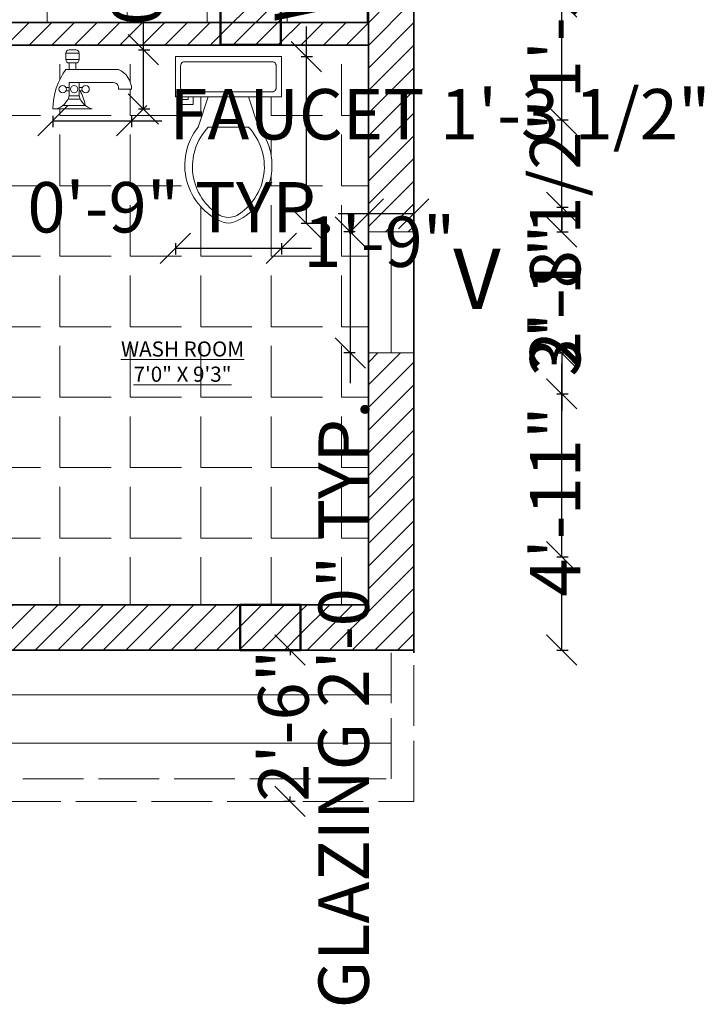
# Model space of a CAD drawing. Units: inches. Extents: x 2036 to 2670, y 319 to 920.
# Tile 13 of 15: x 2535 to 2670, y 424 to 620. Entities that reach past the tile are written whole.
import ezdxf

# ---------------------------------------------------------------- set-up
doc = ezdxf.new("R2010")
doc.units = ezdxf.units.IN
doc.linetypes.add('ACAD_ISO02W100', pattern=[15, 12, -3])
for name, color, linetype, lineweight in [('A-ANNO-DIMS', 2, 'Continuous', 18), ('A-ANNO-TEXT', 7, 'Continuous', 18), ('A-AREA-IDEN', 7, 'Continuous', 18), ('A-COLS', 7, 'Continuous', 50), ('A-FLOR-FIXT', 8, 'Continuous', 18), ('A-FLOR-OVHD', 1, 'ACAD_ISO02W100', 13), ('A-FLOR-PATT', 8, 'Continuous', 9), ('A-GLAZ', 4, 'Continuous', 18), ('A-WALL', 7, 'Continuous', 35)]:
    doc.layers.add(name, color=color, linetype=linetype, lineweight=lineweight)
doc.layers.add('A-COLS-PATT', color=240, linetype='Continuous', lineweight=13, true_color=0xed1f24)
doc.layers.add('A-WALL-PATT', color=52, linetype='Continuous', lineweight=13, true_color=0xc8c92d)
doc.styles.get("Standard").update_dxf_attribs({"font": 'arial.ttf'})
doc.dimstyles.new('ISO-25', dxfattribs={"dimtxt": 10, "dimasz": 6, "dimexe": 1.25, "dimexo": 0.625, "dimtad": 0, "dimdec": 1, "dimlunit": 3, "dimtxsty": 'Standard', "dimblk": 'OBLIQUE', "dimcen": 2.5, "dimclrd": 94, "dimclre": 94, "dimclrt": 1, "dimadec": 0, "dimazin": 0, "dimtfac": 1, "dimtdec": 1, "dimtmove": 0, "dimatfit": 3, "dimfxl": 1, "dimfxlon": 1, "dimarcsym": 0})

# ---------------------------------------------------------------- blocks, each defined once
blk = doc.blocks.new('Toilet - top')
for p, q in [((9.5, -6), (9.5, -2)), ((-10, -8.5), (-8, -8.5)), ((-10, -9.5), (-10, -8.5)), ((-7, -9.5), (-10, -9.5)), ((-8, -8.5), (-8, -8)), ((-7, -8), (-7, -9.5)), ((-4, -8), (-6, -14)), ((4, -8), (6, -14)), ((4, -14), (-4, -14))]:
    blk.add_line(p, q)
blk.add_lwpolyline([(10.5, -8), (10.5, 0), (-10.5, 0), (-10.5, -8)], close=True)
for points in [[(8.5, -1), (-8.5, -1)], [(-9.5, -2), (-9.5, -6)], [(-8.5, -7), (8.5, -7)]]:
    blk.add_lwpolyline(points)
for centre, radius, start, end in [((-8.62, -1.88), 0.884, 81.8699, 188.1301), ((8.62, -1.88), 0.884, 351.8699, 98.1301), ((-8.62, -6.12), 0.884, 171.8699, 278.1301), ((8.62, -6.12), 0.884, 261.8699, 8.1301), ((3.52, -21.58), 12.17, 141.4691, 247.9714), ((4.2, -21.82), 11.33, 136.3677, 238.9468), ((-3.52, -21.58), 12.17, 292.0284, 38.5307), ((-4.2, -21.82), 11.33, 301.053, 43.6321), ((0, -27.88), 4, 245.7318, 294.2682), ((0, -29), 4, 254.8605, 285.1395)]:
    blk.add_arc(centre, radius, start, end)
blk = doc.blocks.new('Faucet - Bathroom side')
for p, q in [((-0.625, 4.25), (0.375, 4.25)), ((0.375, 3.75), (-0.625, 3.75)), ((-0.625, 3), (3.375, 3)), ((-0.375, 3), (-0.375, 3.5)), ((0.125, 3.5), (0.125, 3)), ((-0.375, 1.625), (-0.625, 1.625)), ((2.875, 2), (0.375, 2)), ((0.375, 1.625), (0.625, 1.625)), ((4.375, 1.5), (3.375, 1.5)), ((-0.375, 1.375), (-0.625, 1.375)), ((0.48078, 0.75), (-0.47286, 0.75)), ((0.375, 1.375), (0.625, 1.375)), ((-1.625, 0), (-1.375, 0)), ((-1.375, 0), (1.375, 0)), ((-0.88366, 0.25), (0.88424, 0.25))]:
    blk.add_line(p, q)
for points in [[(-0.375, 4.5), (0.125, 4.5)], [(-0.625, 3.75), (-0.625, 4.25)], [(0.375, 4.25), (0.375, 3.75)], [(0.125, 3.5), (-0.375, 3.5)]]:
    blk.add_lwpolyline(points)
blk.add_lwpolyline([(-0.375, 1), (-0.375, 2), (0.375, 2), (0.375, 1)], close=True)
for centre in [(-0.875, 1.5), (0, 1.5), (0.875, 1.5)]:
    blk.add_circle(centre, 0.27951)
for centre, radius, start, end in [((-0.38253, 4.2575), 0.24259, 88.22243, 181.7776), ((0.13252, 4.2575), 0.24259, 358.2224, 91.77757), ((-0.38253, 3.7424), 0.24259, 178.2224, 271.7776), ((0.13252, 3.7424), 0.24259, 268.2224, 1.777565), ((3.45929, -0.0281), 5.08436, 143.4467, 179.6834), ((2.70708, 1.4714), 1.66816, 0.9827695, 66.39737), ((2.96867, 1.5936), 0.41699, 347.0192, 102.9808), ((-1.75, 1.375), 1.42522, 285.2551, 344.7449), ((1.75, 1.375), 1.42522, 195.2551, 254.7449), ((-2.49562, -0.286), 3.38273, 9.709485, 29.48735)]:
    blk.add_arc(centre, radius, start, end)
blk = doc.blocks.new('_Oblique')
at = {"color": 0, "linetype": 'ByBlock', "lineweight": -2}
blk.add_line((-0.5, -0.5), (0.5, 0.5), dxfattribs=at)
blk = doc.blocks.new('*D12')
at = {"layer": 'A-ANNO-DIMS', "color": 0, "lineweight": -2, "transparency": 16777216}
for p, q in [((2589.2, 494.68), (2586.95, 494.68)), ((2588.2, 494.68), (2588.2, 493.69)), ((2588.2, 464.68), (2588.2, 465.68)), ((2589.2, 464.68), (2586.95, 464.68))]:
    blk.add_line(p, q, dxfattribs=at)
at = {"layer": 'Defpoints', "color": 0, "transparency": 16777216}
for p in [(2588.2, 494.68), (2612.74, 494.68), (2612.74, 464.68)]:
    blk.add_point(p, dxfattribs=at)
at = {"layer": 'A-ANNO-DIMS', "color": 0, "lineweight": -2, "transparency": 16777216, "xscale": 6, "yscale": 6, "zscale": 6}
for p, rotation in [((2588.2, 494.68), 90), ((2588.2, 464.68), 270)]:
    blk.add_blockref('_Oblique', p, dxfattribs=dict(at, rotation=rotation))
at = {"layer": 'A-ANNO-DIMS', "color": 0, "transparency": 16777216, "insert": (2588.2, 479.68), "char_height": 10, "attachment_point": 5, "rotation": 90}
blk.add_mtext('2\'-6"', dxfattribs=at)
blk = doc.blocks.new('COL-9x12')
blk.add_lwpolyline([(9, 0), (0, 0), (0, 12), (9, 12)], close=True)
blk = doc.blocks.new('GLAZ-24x9-PLAN')
for p, q in [((9, 24), (0, 24)), ((4.5, 24), (4.5, 0)), ((9, 0), (0, 0))]:
    blk.add_line(p, q)
blk = doc.blocks.new('*D29')
at = {"layer": 'A-ANNO-DIMS', "color": 94, "lineweight": -2, "transparency": 16777216}
for p, q in [((2601.14, 577.61), (2598.89, 577.61)), ((2600.14, 577.61), (2600.14, 553.61)), ((2601.14, 553.61), (2598.89, 553.61)), ((2600.14, 553.61), (2600.14, 547.61))]:
    blk.add_line(p, q, dxfattribs=at)
at = {"layer": 'Defpoints', "color": 0, "transparency": 16777216}
for p in [(2603.74, 577.61), (2600.14, 553.61), (2603.74, 553.61)]:
    blk.add_point(p, dxfattribs=at)
at = {"layer": 'A-ANNO-DIMS', "color": 94, "lineweight": -2, "transparency": 16777216, "xscale": 6, "yscale": 6, "zscale": 6}
for p, rotation in [((2600.14, 577.61), 90), ((2600.14, 553.61), 270)]:
    blk.add_blockref('_Oblique', p, dxfattribs=dict(at, rotation=rotation))
at = {"layer": 'A-ANNO-DIMS', "color": 1, "transparency": 16777216, "insert": (2600.14, 483.98), "char_height": 10, "attachment_point": 5, "rotation": 90}
blk.add_mtext('GLAZING 2\'-0" TYP.', dxfattribs=at)
blk = doc.blocks.new('*D30')
at = {"layer": 'A-ANNO-DIMS', "color": 94, "lineweight": -2, "transparency": 16777216}
for p, q in [((2603.74, 580.21), (2603.74, 582.46)), ((2612.74, 580.21), (2612.74, 582.46)), ((2603.74, 581.21), (2597.74, 581.21)), ((2612.74, 581.21), (2603.74, 581.21))]:
    blk.add_line(p, q, dxfattribs=at)
at = {"layer": 'Defpoints', "color": 0, "transparency": 16777216}
for p in [(2603.74, 581.21), (2603.74, 577.61), (2612.74, 577.61)]:
    blk.add_point(p, dxfattribs=at)
at = {"layer": 'A-ANNO-DIMS', "color": 94, "lineweight": -2, "transparency": 16777216, "xscale": 6, "yscale": 6, "zscale": 6, "rotation": 180}
blk.add_blockref('_Oblique', (2603.74, 581.21), dxfattribs=at)
at = {"layer": 'A-ANNO-DIMS', "color": 94, "lineweight": -2, "transparency": 16777216, "xscale": 6, "yscale": 6, "zscale": 6}
blk.add_blockref('_Oblique', (2612.74, 581.21), dxfattribs=at)
at = {"layer": 'A-ANNO-DIMS', "color": 1, "transparency": 16777216, "insert": (2566.63, 581.21), "char_height": 10, "attachment_point": 5}
blk.add_mtext('0\'-9" TYP.', dxfattribs=at)
blk = doc.blocks.new('*D35')
at = {"layer": 'A-ANNO-DIMS', "color": 94, "lineweight": -2, "transparency": 16777216}
for p, q in [((2591.44, 612.38), (2591.44, 618.38)), ((2590.44, 612.38), (2592.69, 612.38)), ((2591.44, 579.34), (2591.44, 612.38)), ((2590.44, 579.34), (2592.69, 579.34))]:
    blk.add_line(p, q, dxfattribs=at)
at = {"layer": 'Defpoints', "color": 0, "transparency": 16777216}
for p in [(2586.48, 612.38), (2591.44, 612.38), (2586.48, 579.34)]:
    blk.add_point(p, dxfattribs=at)
at = {"layer": 'A-ANNO-DIMS', "color": 94, "lineweight": -2, "transparency": 16777216, "xscale": 6, "yscale": 6, "zscale": 6}
for p, rotation in [((2591.44, 612.38), 90), ((2591.44, 579.34), 270)]:
    blk.add_blockref('_Oblique', p, dxfattribs=dict(at, rotation=rotation))
at = {"layer": 'A-ANNO-DIMS', "color": 1, "transparency": 16777216, "insert": (2591.44, 646.08), "char_height": 10, "attachment_point": 5, "rotation": 90}
blk.add_mtext('WC 2\'-9"', dxfattribs=at)
blk = doc.blocks.new('*D36')
at = {"layer": 'A-ANNO-DIMS', "color": 94, "lineweight": -2, "transparency": 16777216}
for p, q in [((2565.48, 575.38), (2565.48, 573.13)), ((2565.48, 574.38), (2586.48, 574.38)), ((2586.48, 575.38), (2586.48, 573.13)), ((2586.48, 574.38), (2592.48, 574.38))]:
    blk.add_line(p, q, dxfattribs=at)
at = {"layer": 'Defpoints', "color": 0, "transparency": 16777216}
for p in [(2565.48, 579.34), (2586.48, 579.34), (2586.48, 574.38)]:
    blk.add_point(p, dxfattribs=at)
at = {"layer": 'A-ANNO-DIMS', "color": 94, "lineweight": -2, "transparency": 16777216, "xscale": 6, "yscale": 6, "zscale": 6, "rotation": 180}
blk.add_blockref('_Oblique', (2565.48, 574.38), dxfattribs=at)
at = {"layer": 'A-ANNO-DIMS', "color": 94, "lineweight": -2, "transparency": 16777216, "xscale": 6, "yscale": 6, "zscale": 6}
blk.add_blockref('_Oblique', (2586.48, 574.38), dxfattribs=at)
at = {"layer": 'A-ANNO-DIMS', "color": 1, "transparency": 16777216, "insert": (2605.93, 574.38), "char_height": 10, "attachment_point": 5}
blk.add_mtext('1\'-9"', dxfattribs=at)
blk = doc.blocks.new('*D37')
at = {"layer": 'A-ANNO-DIMS', "color": 94, "lineweight": -2, "transparency": 16777216}
for p, q in [((2541.16, 600.66), (2541.16, 598.41)), ((2541.16, 599.66), (2556.79, 599.66)), ((2556.79, 600.66), (2556.79, 598.41)), ((2556.79, 599.66), (2562.79, 599.66))]:
    blk.add_line(p, q, dxfattribs=at)
at = {"layer": 'Defpoints', "color": 0, "transparency": 16777216}
for p in [(2541.16, 602.01), (2556.79, 602.01), (2556.79, 599.66)]:
    blk.add_point(p, dxfattribs=at)
at = {"layer": 'A-ANNO-DIMS', "color": 94, "lineweight": -2, "transparency": 16777216, "xscale": 6, "yscale": 6, "zscale": 6, "rotation": 180}
blk.add_blockref('_Oblique', (2541.16, 599.66), dxfattribs=at)
at = {"layer": 'A-ANNO-DIMS', "color": 94, "lineweight": -2, "transparency": 16777216, "xscale": 6, "yscale": 6, "zscale": 6}
blk.add_blockref('_Oblique', (2556.79, 599.66), dxfattribs=at)
at = {"layer": 'A-ANNO-DIMS', "color": 1, "transparency": 16777216, "insert": (2617.95, 599.66), "char_height": 10, "attachment_point": 5}
blk.add_mtext('FAUCET 1\'-3 1/2"', dxfattribs=at)
blk = doc.blocks.new('*D38')
at = {"layer": 'A-ANNO-DIMS', "color": 94, "lineweight": -2, "transparency": 16777216}
for p, q in [((2559.13, 613.74), (2559.13, 619.74)), ((2558.13, 613.74), (2560.38, 613.74)), ((2559.13, 602.01), (2559.13, 613.74)), ((2558.13, 602.01), (2560.38, 602.01))]:
    blk.add_line(p, q, dxfattribs=at)
at = {"layer": 'Defpoints', "color": 0, "transparency": 16777216}
for p in [(2556.79, 613.74), (2559.13, 613.74), (2556.79, 602.01)]:
    blk.add_point(p, dxfattribs=at)
at = {"layer": 'A-ANNO-DIMS', "color": 94, "lineweight": -2, "transparency": 16777216, "xscale": 6, "yscale": 6, "zscale": 6}
for p, rotation in [((2559.13, 613.74), 90), ((2559.13, 602.01), 270)]:
    blk.add_blockref('_Oblique', p, dxfattribs=dict(at, rotation=rotation))
at = {"layer": 'A-ANNO-DIMS', "color": 1, "transparency": 16777216, "insert": (2559.13, 649.19), "char_height": 10, "attachment_point": 5, "rotation": 90}
blk.add_mtext('0\'-11 1/2"', dxfattribs=at)
blk = doc.blocks.new('*D45')
at = {"layer": 'A-ANNO-DIMS', "color": 94, "lineweight": -2, "transparency": 16777216}
for p, q in [((2641.09, 553.61), (2643.34, 553.61)), ((2642.09, 553.61), (2642.09, 542.15)), ((2642.09, 494.68), (2642.09, 506.14)), ((2641.09, 494.68), (2643.34, 494.68))]:
    blk.add_line(p, q, dxfattribs=at)
at = {"layer": 'Defpoints', "color": 0, "transparency": 16777216}
for p in [(2612.74, 553.61), (2642.09, 553.61), (2612.74, 494.68)]:
    blk.add_point(p, dxfattribs=at)
at = {"layer": 'A-ANNO-DIMS', "color": 94, "lineweight": -2, "transparency": 16777216, "xscale": 6, "yscale": 6, "zscale": 6}
for p, rotation in [((2642.09, 553.61), 90), ((2642.09, 494.68), 270)]:
    blk.add_blockref('_Oblique', p, dxfattribs=dict(at, rotation=rotation))
at = {"layer": 'A-ANNO-DIMS', "color": 1, "transparency": 16777216, "insert": (2642.09, 524.15), "char_height": 10, "attachment_point": 5, "rotation": 90}
blk.add_mtext('4\'-11"', dxfattribs=at)
blk = doc.blocks.new('*D46')
at = {"layer": 'A-ANNO-DIMS', "color": 94, "lineweight": -2, "transparency": 16777216}
for p, q in [((2642.09, 623.23), (2642.09, 629.23)), ((2641.09, 623.23), (2643.34, 623.23)), ((2642.09, 577.61), (2642.09, 623.23)), ((2641.09, 577.61), (2643.34, 577.61))]:
    blk.add_line(p, q, dxfattribs=at)
at = {"layer": 'Defpoints', "color": 0, "transparency": 16777216}
for p in [(2612.74, 623.23), (2642.09, 623.23), (2612.74, 577.61)]:
    blk.add_point(p, dxfattribs=at)
at = {"layer": 'A-ANNO-DIMS', "color": 94, "lineweight": -2, "transparency": 16777216, "xscale": 6, "yscale": 6, "zscale": 6}
for p, rotation in [((2642.09, 623.23), 90), ((2642.09, 577.61), 270)]:
    blk.add_blockref('_Oblique', p, dxfattribs=dict(at, rotation=rotation))
at = {"layer": 'A-ANNO-DIMS', "color": 1, "transparency": 16777216, "insert": (2642.09, 654.79), "char_height": 10, "attachment_point": 5, "rotation": 90}
blk.add_mtext('3\'-9 1/2"', dxfattribs=at)
blk = doc.blocks.new('*D54')
at = {"layer": 'A-ANNO-DIMS', "color": 94, "lineweight": -2, "transparency": 16777216}
for p, q in [((2642.09, 545.51), (2642.09, 551.51)), ((2641.09, 545.51), (2643.34, 545.51)), ((2642.09, 513.19), (2642.09, 545.51)), ((2641.09, 513.19), (2643.34, 513.19))]:
    blk.add_line(p, q, dxfattribs=at)
at = {"layer": 'Defpoints', "color": 0, "transparency": 16777216}
for p in [(2158.74, 545.51), (2642.09, 545.51), (2158.74, 513.19)]:
    blk.add_point(p, dxfattribs=at)
at = {"layer": 'A-ANNO-DIMS', "color": 94, "lineweight": -2, "transparency": 16777216, "xscale": 6, "yscale": 6, "zscale": 6}
for p, rotation in [((2642.09, 545.51), 90), ((2642.09, 513.19), 270)]:
    blk.add_blockref('_Oblique', p, dxfattribs=dict(at, rotation=rotation))
at = {"layer": 'A-ANNO-DIMS', "color": 1, "transparency": 16777216, "insert": (2642.09, 577.16), "char_height": 10, "attachment_point": 5, "rotation": 90}
blk.add_mtext('2\'-8 1/2"', dxfattribs=at)
blk = doc.blocks.new('*D55')
at = {"layer": 'A-ANNO-DIMS', "color": 94, "lineweight": -2, "transparency": 16777216}
for p, q in [((2641.09, 582.53), (2643.34, 582.53)), ((2642.09, 582.53), (2642.09, 577.94)), ((2642.09, 545.51), (2642.09, 550.11)), ((2641.09, 545.51), (2643.34, 545.51))]:
    blk.add_line(p, q, dxfattribs=at)
at = {"layer": 'Defpoints', "color": 0, "transparency": 16777216}
for p in [(2158.74, 582.53), (2642.09, 582.53), (2158.74, 545.51)]:
    blk.add_point(p, dxfattribs=at)
at = {"layer": 'A-ANNO-DIMS', "color": 94, "lineweight": -2, "transparency": 16777216, "xscale": 6, "yscale": 6, "zscale": 6}
for p, rotation in [((2642.09, 582.53), 90), ((2642.09, 545.51), 270)]:
    blk.add_blockref('_Oblique', p, dxfattribs=dict(at, rotation=rotation))
at = {"layer": 'A-ANNO-DIMS', "color": 1, "transparency": 16777216, "insert": (2642.09, 564.02), "char_height": 10, "attachment_point": 5, "rotation": 90}
blk.add_mtext('3\'-1"', dxfattribs=at)
blk = doc.blocks.new('*D56')
at = {"layer": 'A-ANNO-DIMS', "color": 94, "lineweight": -2, "transparency": 16777216}
for p, q in [((2642.09, 599.85), (2642.09, 605.85)), ((2641.09, 599.85), (2643.34, 599.85)), ((2642.09, 582.53), (2642.09, 599.85)), ((2641.09, 582.53), (2643.34, 582.53))]:
    blk.add_line(p, q, dxfattribs=at)
at = {"layer": 'Defpoints', "color": 0, "transparency": 16777216}
for p in [(2158.74, 599.85), (2642.09, 599.85), (2158.74, 582.53)]:
    blk.add_point(p, dxfattribs=at)
at = {"layer": 'A-ANNO-DIMS', "color": 94, "lineweight": -2, "transparency": 16777216, "xscale": 6, "yscale": 6, "zscale": 6}
for p, rotation in [((2642.09, 599.85), 90), ((2642.09, 582.53), 270)]:
    blk.add_blockref('_Oblique', p, dxfattribs=dict(at, rotation=rotation))
at = {"layer": 'A-ANNO-DIMS', "color": 1, "transparency": 16777216, "insert": (2642.09, 630.95), "char_height": 10, "attachment_point": 5, "rotation": 90}
blk.add_mtext('1\'-5 1/2"', dxfattribs=at)

msp = doc.modelspace()

# ---------------------------------------------------------------- hatches: boundary and pattern name
at = {"layer": 'A-COLS-PATT'}
h = msp.add_hatch(dxfattribs=at)
h.set_pattern_fill('ANSI31', color=256)
h.paths.add_polyline_path([(2089.74, 875.68), (2080.74, 875.68), (2080.74, 863.68), (2089.74, 863.68)])
h.paths.add_polyline_path([(2089.74, 821.68), (2080.74, 821.68), (2080.74, 809.68), (2089.74, 809.68)])
h.paths.add_polyline_path([(2089.74, 624.2), (2080.74, 624.2), (2080.74, 612.2), (2089.74, 612.2)])
h.paths.add_polyline_path([(2158.74, 506.68), (2149.74, 506.68), (2149.74, 494.68), (2158.74, 494.68)])
h.paths.add_polyline_path([(2158.74, 617.33), (2149.74, 617.33), (2149.74, 605.33), (2158.74, 605.33)])
h.paths.add_polyline_path([(2158.74, 736.18), (2149.74, 736.18), (2149.74, 724.18), (2158.74, 724.18)])
h.paths.add_polyline_path([(2158.74, 852.81), (2149.74, 852.81), (2149.74, 843.81), (2158.74, 843.81)])
h.paths.add_polyline_path([(2161.74, 852.81), (2158.74, 852.81), (2158.74, 843.81), (2161.74, 843.81)])
h.paths.add_polyline_path([(2295.21, 857.66), (2290.74, 857.66), (2290.74, 848.68), (2295.21, 848.68)])
h.paths.add_polyline_path([(2290.74, 857.66), (2283.21, 857.66), (2283.21, 848.66), (2290.74, 848.66)])
h.paths.add_polyline_path([(2443.62, 857.68), (2431.62, 857.68), (2431.62, 848.68), (2443.62, 848.68)])
h.paths.add_polyline_path([(2561.81, 857.68), (2549.81, 857.68), (2549.81, 848.68), (2561.81, 848.68)])
h.paths.add_polyline_path([(2295.24, 737.65), (2290.74, 737.65), (2290.74, 728.68), (2295.24, 728.68)])
h.paths.add_polyline_path([(2309.27, 612.12), (2297.27, 612.12), (2297.27, 603.12), (2309.27, 603.12)])
h.paths.add_polyline_path([(2282.24, 503.68), (2270.24, 503.68), (2270.24, 494.68), (2282.24, 494.68)])
h.paths.add_polyline_path([(2431.74, 746.09), (2427.24, 746.09), (2427.24, 737.09), (2431.74, 737.09)])
h.paths.add_polyline_path([(2439.24, 746.09), (2431.74, 746.09), (2431.74, 737.09), (2439.24, 737.09)])
h.paths.add_polyline_path([(2596.59, 736.59), (2584.59, 736.59), (2584.59, 727.59), (2596.59, 727.59)])
h.paths.add_polyline_path([(2586.39, 623.71), (2574.39, 623.71), (2574.39, 619.18), (2586.39, 619.18)])
h.paths.add_polyline_path([(2586.39, 619.18), (2574.39, 619.18), (2574.39, 614.71), (2586.39, 614.71)])
h.paths.add_polyline_path([(2438.74, 623.68), (2431.24, 623.68), (2431.24, 619.18), (2438.74, 619.18)])
h.paths.add_polyline_path([(2438.74, 619.18), (2431.24, 619.18), (2431.24, 614.68), (2438.74, 614.68)])
h.paths.add_polyline_path([(2431.24, 623.68), (2426.74, 623.68), (2426.74, 614.68), (2431.24, 614.68), (2431.24, 619.18)])
h.paths.add_polyline_path([(2527.24, 503.68), (2515.24, 503.68), (2515.24, 494.68), (2527.24, 494.68)])
h.paths.add_polyline_path([(2590.31, 503.68), (2578.31, 503.68), (2578.31, 494.68), (2590.31, 494.68)])
at = {"layer": 'A-FLOR-PATT'}
h = msp.add_hatch(dxfattribs=at)
h.set_pattern_fill('ANSI31', color=256, scale=5, angle=135)
h.paths.add_polyline_path([(2290.74, 659.68), (2158.74, 659.68), (2158.74, 582.53), (2158.74, 545.51), (2158.74, 503.68), (2426.74, 503.68), (2426.74, 614.68), (2426.74, 623.68), (2426.74, 628.18), (2431.24, 628.18), (2431.24, 623.68), (2438.74, 623.68), (2438.74, 619.18), (2574.39, 619.18), (2574.39, 623.71), (2586.39, 623.71), (2586.39, 619.18), (2603.74, 619.18), (2603.74, 824.68), (2431.74, 824.68), (2431.74, 746.09), (2439.24, 746.09), (2439.24, 737.09), (2431.74, 737.09), (2431.74, 659.68), (2427.24, 659.68), (2427.24, 739.48), (2383.24, 739.48), (2383.24, 804.68), (2339.24, 804.68), (2339.24, 749.08), (2295.24, 749.08), (2295.24, 737.65), (2295.27, 737.65), (2295.27, 728.65), (2295.21, 728.65, -0.586418), (2272.74, 728.68), (2272.74, 824.68), (2270.11, 824.68), (2270.11, 829.18), (2290.74, 829.18), (2290.74, 848.66), (2283.21, 848.66), (2283.21, 857.66), (2289.74, 857.66), (2289.74, 874.68), (2158.74, 874.68), (2158.74, 852.81), (2161.74, 852.81), (2161.74, 843.81), (2158.74, 843.81), (2158.74, 829.18), (2224.74, 829.18), (2224.74, 800.68), (2182.74, 800.68), (2182.74, 733.41), (2158.74, 733.41), (2158.74, 728.68), (2235.24, 728.68), (2235.24, 714.81), (2230.74, 714.81), (2230.74, 724.18), (2158.74, 724.18), (2158.74, 664.18), (2230.74, 664.18), (2230.74, 678.81), (2235.24, 678.81), (2235.24, 664.18), (2290.74, 664.18)])
h.paths.add_polyline_path([(2309.27, 612.12), (2309.27, 603.12), (2297.27, 603.12), (2297.27, 612.12)], flags=16)
h.paths.add_polyline_path([(2280.12, 639.11), (2280.26, 638.18, -0.414214), (2279.26, 637.18), (2278.76, 637.18), (2279.26, 633.18), (2277.76, 633.18), (2277.26, 637.18), (2269.76, 637.18), (2262.26, 637.18), (2261.76, 633.18), (2260.26, 633.18), (2260.76, 637.18), (2260.26, 637.18, -0.414214), (2259.26, 638.18), (2259.41, 639.11, -0.541164), (2257.76, 641.18), (2260.76, 652.18), (2261.45, 652.18), (2261.53, 652.68), (2262.76, 652.68), (2262.25, 655.24, 0.001913), (2261.76, 655.18), (2259.76, 658.18, -0.15), (2279.76, 658.18), (2277.76, 655.18, 0.001913), (2277.27, 655.24), (2276.76, 652.68), (2278, 652.68), (2278.07, 652.18), (2278.76, 652.18), (2281.76, 641.18, -0.541163)], flags=16)
h.paths.add_polyline_path([(2245.98, 639.11), (2246.13, 638.18, -0.414214), (2245.13, 637.18), (2244.63, 637.18), (2245.13, 633.18), (2243.63, 633.18), (2243.13, 637.18), (2235.63, 637.18), (2228.13, 637.18), (2227.63, 633.18), (2226.13, 633.18), (2226.63, 637.18), (2226.13, 637.18, -0.414214), (2225.13, 638.18), (2225.27, 639.11, -0.541164), (2223.63, 641.18), (2226.63, 652.18), (2227.32, 652.18), (2227.39, 652.68), (2228.63, 652.68), (2228.12, 655.24, 0.001913), (2227.63, 655.18), (2225.63, 658.18, -0.15), (2245.63, 658.18), (2243.63, 655.18, 0.001913), (2243.14, 655.24), (2242.63, 652.68), (2243.86, 652.68), (2243.94, 652.18), (2244.63, 652.18), (2247.63, 641.18, -0.541163)], flags=16)
h.paths.add_polyline_path([(2351.59, 515.15, -0.151948), (2279.59, 515.15), (2279.59, 537.68), (2273.59, 537.68), (2273.59, 511.68, 0.190476), (2357.59, 511.68), (2357.59, 537.68), (2351.59, 537.68)])
h.paths.add_polyline_path([(2327.59, 536.13), (2327.59, 517.07), (2303.59, 517.07), (2303.59, 536.13)], flags=16)
h.paths.add_polyline_path([(2213.4, 639.11), (2213.55, 638.18, -0.414214), (2212.55, 637.18), (2212.05, 637.18), (2212.55, 633.18), (2211.05, 633.18), (2210.55, 637.18), (2203.05, 637.18), (2195.55, 637.18), (2195.05, 633.18), (2193.55, 633.18), (2194.05, 637.18), (2193.55, 637.18, -0.414214), (2192.55, 638.18), (2192.69, 639.11, -0.541164), (2191.05, 641.18), (2194.05, 652.18), (2194.73, 652.18), (2194.81, 652.68), (2196.05, 652.68), (2195.53, 655.24, 0.001913), (2195.05, 655.18), (2193.05, 658.18, -0.15), (2213.05, 658.18), (2211.05, 655.18, 0.001913), (2210.56, 655.24), (2210.05, 652.68), (2211.28, 652.68), (2211.36, 652.18), (2212.05, 652.18), (2215.05, 641.18, -0.541163)], flags=16)
h.paths.add_polyline_path([(2368.58, 538.02), (2370.52, 538.02), (2371.17, 532.84), (2380.89, 532.84), (2390.6, 532.84), (2391.25, 538.02), (2393.2, 538.02), (2392.55, 532.84), (2380.89, 532.84), (2368.58, 532.84, 0.414214), (2367.28, 531.54), (2367.47, 530.34, -0.483352), (2369.23, 527.65), (2371.82, 513.4), (2370.12, 513.4), (2370.22, 512.75), (2391.56, 512.75), (2391.66, 513.4), (2389.96, 513.4), (2392.55, 527.65, -1.387427), (2396.43, 527.65), (2392.55, 513.4), (2391.66, 513.4), (2391.56, 512.75), (2389.31, 512.75), (2390, 509.37, 0.003796), (2391.25, 509.51), (2393.84, 505.63, -0.15), (2367.93, 505.63), (2370.52, 509.51, 0.003901), (2371.81, 509.36), (2372.47, 512.75), (2370.22, 512.75), (2370.12, 513.4), (2369.23, 513.4), (2365.34, 527.65, -0.541163), (2367.47, 530.34), (2367.28, 531.54, -0.414214), (2368.58, 532.84), (2369.23, 532.84)])
h.paths.add_polyline_path([(2266.74, 538.02), (2266.09, 532.84), (2254.43, 532.84), (2242.12, 532.84, 0.414214), (2240.83, 531.54), (2241.01, 530.34, -0.483352), (2242.77, 527.65), (2245.36, 513.4), (2243.66, 513.4), (2243.76, 512.75), (2265.1, 512.75), (2265.2, 513.4), (2263.5, 513.4), (2266.09, 527.65, -1.387427), (2269.98, 527.65), (2266.09, 513.4), (2265.2, 513.4), (2265.1, 512.75), (2262.85, 512.75), (2263.54, 509.37, 0.003796), (2264.79, 509.51), (2267.39, 505.63, -0.15), (2241.47, 505.63), (2244.07, 509.51, 0.003901), (2245.36, 509.36), (2246.01, 512.75), (2243.76, 512.75), (2243.66, 513.4), (2242.77, 513.4), (2238.88, 527.65, -0.541163), (2241.01, 530.34), (2240.83, 531.54, -0.414214), (2242.12, 532.84), (2242.77, 532.84), (2242.12, 538.02), (2244.07, 538.02), (2244.71, 532.84), (2254.43, 532.84), (2264.15, 532.84), (2264.79, 538.02)])
h.paths.add_polyline_path([(2185.24, 620.36), (2185.24, 618.86), (2181.24, 618.36), (2181.24, 610.86), (2181.24, 603.36), (2185.24, 602.86), (2185.24, 601.36), (2181.24, 601.86), (2181.24, 601.36, -0.414214), (2180.24, 600.36), (2179.31, 600.5, -0.541164), (2177.24, 598.86), (2166.24, 601.86), (2166.24, 602.54), (2165.74, 602.62), (2165.74, 603.86), (2163.18, 603.34, 0.001913), (2163.24, 602.86), (2160.24, 600.86, -0.15), (2160.24, 620.86), (2163.24, 618.86, 0.001913), (2163.18, 618.37), (2165.74, 617.86), (2165.74, 619.09), (2166.24, 619.17), (2166.24, 619.86), (2177.24, 622.86, -0.541163), (2179.31, 621.21), (2180.24, 621.36, -0.414214), (2181.24, 620.36), (2181.24, 619.86)])
h.paths.add_polyline_path([(2470.92, 676.01), (2470.92, 806.13), (2568.52, 806.13), (2568.52, 676.01)], flags=16)
h.paths.add_polyline_path([(2177.74, 677.49), (2161.9, 677.49), (2161.9, 705.85), (2177.74, 705.85)], flags=16)
h.paths.add_polyline_path([(2176.74, 678.49), (2162.9, 678.49), (2162.9, 704.85), (2176.74, 704.85)], flags=0)
h.paths.add_polyline_path([(2175.01, 686.48), (2172.93, 686.48), (2172.93, 690.63), (2170.86, 690.63), (2170.86, 686.48), (2164.63, 686.48), (2164.63, 688.56), (2166.71, 688.56), (2168.78, 688.56), (2168.78, 690.63), (2164.63, 690.63), (2164.63, 696.85), (2166.71, 696.85), (2166.71, 692.71), (2168.78, 692.71), (2168.78, 696.85), (2175.01, 696.85), (2175.01, 694.78), (2170.86, 694.78), (2170.86, 692.71), (2175.01, 692.71)], flags=0)
h.paths.add_polyline_path([(2543.79, 782.71), (2483.94, 782.71), (2483.94, 804.18), (2517.77, 804.18), (2517.77, 782.71), (2521.67, 782.71), (2521.67, 804.18), (2555.5, 804.18), (2555.5, 779.45), (2547.05, 779.45), (2568.52, 757.98), (2543.79, 757.98)], flags=0)
h.paths.add_polyline_path([(2584.59, 727.59), (2584.59, 736.59), (2596.59, 736.59), (2596.59, 727.59)], flags=16)
h.paths.add_polyline_path([(2520.45, 647.03), (2553.79, 647.03), (2553.79, 658.23), (2520.45, 658.23)], flags=24)
h.paths.add_polyline_path([(2299.53, 573.74), (2331.71, 573.74), (2331.71, 584.94), (2299.53, 584.94)], flags=24)
h.paths.add_polyline_path([(2191.59, 685.19), (2212.12, 685.19), (2212.12, 696.38), (2191.59, 696.38)], flags=24)
h.paths.add_polyline_path([(2353.9, 649.86), (2379.08, 649.86), (2379.08, 661.06), (2353.9, 661.06)], flags=24)
h.paths.add_polyline_path([(2214.61, 763.31), (2237.46, 763.31), (2237.46, 779.56), (2214.61, 779.56)], flags=24)
h.paths.add_polyline_path([(2225.09, 819.31), (2269.29, 819.31), (2269.29, 844.04), (2225.09, 844.04)], flags=24)
h.paths.add_polyline_path([(2204.06, 845.04), (2226.92, 845.04), (2226.92, 856.24), (2204.06, 856.24)], flags=24)
h = msp.add_hatch(dxfattribs=at)
h.set_pattern_fill('ANSI31', color=256, scale=5, angle=45)
h.paths.add_polyline_path([(2290.74, 659.68), (2158.74, 659.68), (2158.74, 582.53), (2158.74, 545.51), (2158.74, 503.68), (2426.74, 503.68), (2426.74, 614.68), (2426.74, 623.68), (2426.74, 628.18), (2431.24, 628.18), (2431.24, 623.68), (2438.74, 623.68), (2438.74, 619.18), (2574.39, 619.18), (2574.39, 623.71), (2586.39, 623.71), (2586.39, 619.18), (2603.74, 619.18), (2603.74, 824.68), (2431.74, 824.68), (2431.74, 746.09), (2439.24, 746.09), (2439.24, 737.09), (2431.74, 737.09), (2431.74, 659.68), (2427.24, 659.68), (2427.24, 739.48), (2383.24, 739.48), (2383.24, 804.68), (2339.24, 804.68), (2339.24, 749.08), (2295.24, 749.08), (2295.24, 737.65), (2295.27, 737.65), (2295.27, 728.65), (2295.21, 728.65, -0.586418), (2272.74, 728.68), (2272.74, 824.68), (2270.11, 824.68), (2270.11, 829.18), (2290.74, 829.18), (2290.74, 848.66), (2283.21, 848.66), (2283.21, 857.66), (2289.74, 857.66), (2289.74, 874.68), (2158.74, 874.68), (2158.74, 852.81), (2161.74, 852.81), (2161.74, 843.81), (2158.74, 843.81), (2158.74, 829.18), (2224.74, 829.18), (2224.74, 800.68), (2182.74, 800.68), (2182.74, 733.41), (2158.74, 733.41), (2158.74, 728.68), (2235.24, 728.68), (2235.24, 714.81), (2230.74, 714.81), (2230.74, 724.18), (2158.74, 724.18), (2158.74, 664.18), (2230.74, 664.18), (2230.74, 678.81), (2235.24, 678.81), (2235.24, 664.18), (2290.74, 664.18)])
h.paths.add_polyline_path([(2309.27, 612.12), (2309.27, 603.12), (2297.27, 603.12), (2297.27, 612.12)], flags=16)
h.paths.add_polyline_path([(2280.12, 639.11), (2280.26, 638.18, -0.414214), (2279.26, 637.18), (2278.76, 637.18), (2279.26, 633.18), (2277.76, 633.18), (2277.26, 637.18), (2269.76, 637.18), (2262.26, 637.18), (2261.76, 633.18), (2260.26, 633.18), (2260.76, 637.18), (2260.26, 637.18, -0.414214), (2259.26, 638.18), (2259.41, 639.11, -0.541164), (2257.76, 641.18), (2260.76, 652.18), (2261.45, 652.18), (2261.53, 652.68), (2262.76, 652.68), (2262.25, 655.24, 0.001913), (2261.76, 655.18), (2259.76, 658.18, -0.15), (2279.76, 658.18), (2277.76, 655.18, 0.001913), (2277.27, 655.24), (2276.76, 652.68), (2278, 652.68), (2278.07, 652.18), (2278.76, 652.18), (2281.76, 641.18, -0.541163)], flags=16)
h.paths.add_polyline_path([(2245.98, 639.11), (2246.13, 638.18, -0.414214), (2245.13, 637.18), (2244.63, 637.18), (2245.13, 633.18), (2243.63, 633.18), (2243.13, 637.18), (2235.63, 637.18), (2228.13, 637.18), (2227.63, 633.18), (2226.13, 633.18), (2226.63, 637.18), (2226.13, 637.18, -0.414214), (2225.13, 638.18), (2225.27, 639.11, -0.541164), (2223.63, 641.18), (2226.63, 652.18), (2227.32, 652.18), (2227.39, 652.68), (2228.63, 652.68), (2228.12, 655.24, 0.001913), (2227.63, 655.18), (2225.63, 658.18, -0.15), (2245.63, 658.18), (2243.63, 655.18, 0.001913), (2243.14, 655.24), (2242.63, 652.68), (2243.86, 652.68), (2243.94, 652.18), (2244.63, 652.18), (2247.63, 641.18, -0.541163)], flags=16)
h.paths.add_polyline_path([(2351.59, 537.68), (2351.59, 515.15, -0.151948), (2279.59, 515.15), (2279.59, 537.68), (2273.59, 537.68), (2273.59, 511.68, 0.190476), (2357.59, 511.68), (2357.59, 537.68)])
h.paths.add_polyline_path([(2368.58, 538.02), (2370.52, 538.02), (2371.17, 532.84), (2380.89, 532.84), (2390.6, 532.84), (2391.25, 538.02), (2393.2, 538.02), (2392.55, 532.84), (2380.89, 532.84), (2368.58, 532.84, 0.414214), (2367.28, 531.54), (2367.47, 530.34, -0.483352), (2369.23, 527.65), (2371.82, 513.4), (2370.12, 513.4), (2370.22, 512.75), (2391.56, 512.75), (2391.66, 513.4), (2389.96, 513.4), (2392.55, 527.65, -1.387427), (2396.43, 527.65), (2392.55, 513.4), (2391.66, 513.4), (2391.56, 512.75), (2389.31, 512.75), (2390, 509.37, 0.003796), (2391.25, 509.51), (2393.84, 505.63, -0.15), (2367.93, 505.63), (2370.52, 509.51, 0.003901), (2371.81, 509.36), (2372.47, 512.75), (2370.22, 512.75), (2370.12, 513.4), (2369.23, 513.4), (2365.34, 527.65, -0.541163), (2367.47, 530.34), (2367.28, 531.54, -0.414214), (2368.58, 532.84), (2369.23, 532.84)])
h.paths.add_polyline_path([(2327.59, 536.13), (2327.59, 517.07), (2303.59, 517.07), (2303.59, 536.13)], flags=16)
h.paths.add_polyline_path([(2470.92, 676.01), (2470.92, 806.13), (2568.52, 806.13), (2568.52, 676.01)], flags=16)
h.paths.add_polyline_path([(2266.74, 538.02), (2266.09, 532.84), (2254.43, 532.84), (2242.12, 532.84, 0.414214), (2240.83, 531.54), (2241.01, 530.34, -0.483352), (2242.77, 527.65), (2245.36, 513.4), (2243.66, 513.4), (2243.76, 512.75), (2265.1, 512.75), (2265.2, 513.4), (2263.5, 513.4), (2266.09, 527.65, -1.387427), (2269.98, 527.65), (2266.09, 513.4), (2265.2, 513.4), (2265.1, 512.75), (2262.85, 512.75), (2263.54, 509.37, 0.003796), (2264.79, 509.51), (2267.39, 505.63, -0.15), (2241.47, 505.63), (2244.07, 509.51, 0.003901), (2245.36, 509.36), (2246.01, 512.75), (2243.76, 512.75), (2243.66, 513.4), (2242.77, 513.4), (2238.88, 527.65, -0.541163), (2241.01, 530.34), (2240.83, 531.54, -0.414214), (2242.12, 532.84), (2242.77, 532.84), (2242.12, 538.02), (2244.07, 538.02), (2244.71, 532.84), (2254.43, 532.84), (2264.15, 532.84), (2264.79, 538.02)])
h.paths.add_polyline_path([(2213.4, 639.11), (2213.55, 638.18, -0.414214), (2212.55, 637.18), (2212.05, 637.18), (2212.55, 633.18), (2211.05, 633.18), (2210.55, 637.18), (2203.05, 637.18), (2195.55, 637.18), (2195.05, 633.18), (2193.55, 633.18), (2194.05, 637.18), (2193.55, 637.18, -0.414214), (2192.55, 638.18), (2192.69, 639.11, -0.541164), (2191.05, 641.18), (2194.05, 652.18), (2194.73, 652.18), (2194.81, 652.68), (2196.05, 652.68), (2195.53, 655.24, 0.001913), (2195.05, 655.18), (2193.05, 658.18, -0.15), (2213.05, 658.18), (2211.05, 655.18, 0.001913), (2210.56, 655.24), (2210.05, 652.68), (2211.28, 652.68), (2211.36, 652.18), (2212.05, 652.18), (2215.05, 641.18, -0.541163)], flags=16)
h.paths.add_polyline_path([(2185.24, 620.36), (2185.24, 618.86), (2181.24, 618.36), (2181.24, 610.86), (2181.24, 603.36), (2185.24, 602.86), (2185.24, 601.36), (2181.24, 601.86), (2181.24, 601.36, -0.414214), (2180.24, 600.36), (2179.31, 600.5, -0.541164), (2177.24, 598.86), (2166.24, 601.86), (2166.24, 602.54), (2165.74, 602.62), (2165.74, 603.86), (2163.18, 603.34, 0.001913), (2163.24, 602.86), (2160.24, 600.86, -0.15), (2160.24, 620.86), (2163.24, 618.86, 0.001913), (2163.18, 618.37), (2165.74, 617.86), (2165.74, 619.09), (2166.24, 619.17), (2166.24, 619.86), (2177.24, 622.86, -0.541163), (2179.31, 621.21), (2180.24, 621.36, -0.414214), (2181.24, 620.36), (2181.24, 619.86)])
h.paths.add_polyline_path([(2177.74, 677.49), (2161.9, 677.49), (2161.9, 705.85), (2177.74, 705.85)], flags=16)
h.paths.add_polyline_path([(2176.74, 678.49), (2162.9, 678.49), (2162.9, 704.85), (2176.74, 704.85)], flags=0)
h.paths.add_polyline_path([(2175.01, 686.48), (2172.93, 686.48), (2172.93, 690.63), (2170.86, 690.63), (2170.86, 686.48), (2164.63, 686.48), (2164.63, 688.56), (2166.71, 688.56), (2168.78, 688.56), (2168.78, 690.63), (2164.63, 690.63), (2164.63, 696.85), (2166.71, 696.85), (2166.71, 692.71), (2168.78, 692.71), (2168.78, 696.85), (2175.01, 696.85), (2175.01, 694.78), (2170.86, 694.78), (2170.86, 692.71), (2175.01, 692.71)], flags=0)
h.paths.add_polyline_path([(2543.79, 782.71), (2483.94, 782.71), (2483.94, 804.18), (2517.77, 804.18), (2517.77, 782.71), (2521.67, 782.71), (2521.67, 804.18), (2555.5, 804.18), (2555.5, 779.45), (2547.05, 779.45), (2568.52, 757.98), (2543.79, 757.98)], flags=0)
h.paths.add_polyline_path([(2584.59, 727.59), (2584.59, 736.59), (2596.59, 736.59), (2596.59, 727.59)], flags=16)
h.paths.add_polyline_path([(2520.45, 647.03), (2553.79, 647.03), (2553.79, 658.23), (2520.45, 658.23)], flags=24)
h.paths.add_polyline_path([(2299.53, 573.74), (2331.71, 573.74), (2331.71, 584.94), (2299.53, 584.94)], flags=24)
h.paths.add_polyline_path([(2191.59, 685.19), (2212.12, 685.19), (2212.12, 696.38), (2191.59, 696.38)], flags=24)
h.paths.add_polyline_path([(2353.9, 649.86), (2379.08, 649.86), (2379.08, 661.06), (2353.9, 661.06)], flags=24)
h.paths.add_polyline_path([(2214.61, 763.31), (2237.46, 763.31), (2237.46, 779.56), (2214.61, 779.56)], flags=24)
h.paths.add_polyline_path([(2225.09, 819.31), (2269.29, 819.31), (2269.29, 844.04), (2225.09, 844.04)], flags=24)
h.paths.add_polyline_path([(2204.06, 845.04), (2226.92, 845.04), (2226.92, 856.24), (2204.06, 856.24)], flags=24)
h = msp.add_hatch(dxfattribs=at)
h.set_pattern_fill('ANSI31', color=256, scale=3, angle=135)
h.paths.add_polyline_path([(2149.74, 582.53), (2149.74, 707.68), (2120.74, 707.68), (2120.74, 599.68, -1), (2118.74, 599.68), (2085.24, 599.68), (2085.24, 506.68), (2089.74, 506.68), (2089.74, 494.68), (2085.24, 494.68), (2085.24, 469.18), (2608.24, 469.18), (2608.24, 494.68), (2149.74, 494.68), (2149.74, 506.68), (2149.74, 545.51)])
h.paths.add_polyline_path([(2143.58, 686.71), (2149.03, 686.71), (2149.03, 692.89), (2143.58, 692.89)], flags=24)
h.paths.add_polyline_path([(2125.99, 700.31), (2133.31, 700.31), (2133.31, 706.49), (2125.99, 706.49)], flags=24)
h = msp.add_hatch(dxfattribs=at)
h.set_pattern_fill('ANGLE', color=256, scale=2)
h.set_pattern_definition([(0, (0, 0), (0, 13.97), [10.16, -3.81]), (90, (0, 0), (-13.97, 9e-16), [10.16, -3.81])])
h.paths.add_polyline_path([(2519.74, 503.68), (2527.24, 503.68), (2603.74, 503.68), (2603.74, 614.68), (2519.74, 614.68)])
h.paths.add_polyline_path([(2569.98, 598.38), (2571.98, 604.38), (2568.98, 604.38), (2568.98, 602.88), (2565.98, 602.88), (2565.98, 603.88), (2567.98, 603.88), (2567.98, 604.38), (2565.48, 604.38), (2565.48, 612.38), (2586.48, 612.38), (2586.48, 604.38), (2579.98, 604.38), (2581.98, 598.38, -0.501323), (2577.03, 579.52, -0.132891), (2574.94, 579.52, -0.501317)], flags=16)
h.paths.add_polyline_path([(2571.98, 598.38), (2579.98, 598.38, -0.48008), (2577.63, 580.86, -0.215004), (2574.34, 580.86, -0.48008)], flags=0)
h.paths.add_polyline_path([(2546.37, 611.78), (2546.37, 613.08), (2543.76, 613.08), (2543.76, 611.78)], flags=16)
h.paths.add_polyline_path([(2543.76, 609.82), (2544.41, 609.82), (2544.41, 611.13), (2545.72, 611.13), (2545.72, 609.82), (2554.18, 609.82, -0.293434), (2556.79, 605.92), (2554.18, 605.92, 0.553806), (2552.88, 607.22), (2546.37, 607.22), (2546.37, 606.24), (2547.02, 606.24, -0.791418), (2548.4, 605.92, -0.791418), (2547.02, 605.59), (2546.57, 605.59, -0.086626), (2547.58, 602.73, 0.107048), (2548.97, 602.01), (2541.81, 602.01), (2541.16, 602.01, -0.159443)], flags=16)
h.paths.add_polyline_path([(2542.38, 605.92, -1), (2543.84, 605.92, -1)], flags=0)
h.paths.add_polyline_path([(2544.66, 605.92, -1), (2546.12, 605.92, -1)], flags=0)
h.paths.add_polyline_path([(2566.48, 606.38), (2566.48, 610.38, -0.5), (2567.48, 611.38), (2584.48, 611.38, -0.5), (2585.48, 610.38), (2585.48, 606.38, -0.5), (2584.48, 605.38), (2567.48, 605.38, -0.5)], flags=0)
h.paths.add_polyline_path([(2552.87, 546.2), (2581.15, 546.2), (2581.15, 557.39), (2552.87, 557.39)], flags=24)
at = {"layer": 'A-WALL-PATT'}
h = msp.add_hatch(dxfattribs=at)
h.set_pattern_fill('ANSI31', color=256)
h.paths.add_polyline_path([(2089.74, 863.68), (2080.74, 863.68), (2080.74, 821.68), (2089.74, 821.68)])
h.paths.add_polyline_path([(2089.74, 809.68), (2080.74, 809.68), (2080.74, 624.2), (2089.74, 624.2), (2089.74, 707.68), (2089.74, 767.68)])
h.paths.add_polyline_path([(2149.74, 818.68), (2089.74, 818.68), (2089.74, 809.68), (2149.74, 809.68)])
h.paths.add_polyline_path([(2158.74, 875.68), (2089.74, 875.68), (2089.74, 866.68), (2149.74, 866.68), (2149.74, 852.81), (2158.74, 852.81)])
h.paths.add_polyline_path([(2158.74, 843.81), (2149.74, 843.81), (2149.74, 736.18), (2158.74, 736.18), (2158.74, 824.68)])
h.paths.add_polyline_path([(2181.31, 829.18), (2158.74, 829.18), (2158.74, 824.68), (2181.31, 824.68)])
h.paths.add_polyline_path([(2224.74, 829.18), (2212.72, 829.18), (2212.72, 824.68), (2224.74, 824.68)])
h.paths.add_polyline_path([(2177.02, 503.68), (2158.74, 503.68), (2158.74, 494.68), (2177.02, 494.68)])
h.paths.add_polyline_path([(2158.74, 664.18), (2158.74, 680.02), (2149.74, 680.02), (2149.74, 617.33), (2158.74, 617.33)])
h.paths.add_polyline_path([(2158.74, 724.18), (2149.74, 724.18), (2149.74, 704.02), (2158.74, 704.02)])
h.paths.add_polyline_path([(2235.24, 728.68), (2158.74, 728.68), (2158.74, 724.18), (2230.74, 724.18), (2230.74, 714.81), (2235.24, 714.81)])
h.paths.add_polyline_path([(2290.74, 664.18), (2235.24, 664.18), (2235.24, 678.81), (2230.74, 678.81), (2230.74, 664.18), (2158.74, 664.18), (2158.74, 659.68), (2290.74, 659.68)])
h.paths.add_polyline_path([(2270.24, 503.68), (2227.17, 503.68), (2227.17, 494.68), (2270.24, 494.68)])
h.paths.add_polyline_path([(2515.24, 503.68), (2380.89, 503.68), (2380.89, 494.68), (2515.24, 494.68)])
h.paths.add_polyline_path([(2292.21, 503.68), (2282.24, 503.68), (2282.24, 494.68), (2292.21, 494.68)])
h.paths.add_polyline_path([(2578.31, 503.68), (2527.24, 503.68), (2527.24, 494.68), (2578.31, 494.68)])
h.paths.add_polyline_path([(2603.74, 503.68), (2590.31, 503.68), (2590.31, 494.68), (2603.74, 494.68)])
h.paths.add_polyline_path([(2612.74, 503.68), (2603.74, 503.68), (2603.74, 494.68), (2612.74, 494.68)])
h.paths.add_polyline_path([(2549.81, 857.68), (2443.62, 857.68), (2443.62, 848.68), (2549.81, 848.68)])
h.paths.add_polyline_path([(2295.24, 848.66), (2290.74, 848.66), (2290.74, 829.18), (2270.11, 829.18), (2270.11, 824.68), (2290.74, 824.68), (2290.74, 737.65), (2295.24, 737.65)])
h.paths.add_polyline_path([(2431.74, 737.09), (2427.24, 737.09), (2427.24, 659.68), (2431.74, 659.68)])
h.paths.add_polyline_path([(2431.74, 848.68), (2427.24, 848.68), (2427.24, 746.09), (2431.74, 746.09)])
h.paths.add_polyline_path([(2574.39, 619.18), (2495.46, 619.18), (2495.46, 614.68), (2574.39, 614.68)])
h.paths.add_polyline_path([(2461.84, 619.18), (2438.74, 619.18), (2438.74, 614.68), (2461.84, 614.68)])
h.paths.add_polyline_path([(2603.74, 619.18), (2586.39, 619.18), (2586.39, 614.68), (2603.74, 614.68)], flags=17)
h = msp.add_hatch(dxfattribs=at)
h.set_pattern_fill('ANSI31', color=256)
h.paths.add_polyline_path([(2561.81, 857.68), (2561.81, 848.68), (2603.74, 848.68), (2603.74, 798.38), (2612.74, 798.38), (2612.74, 857.68)])
h.paths.add_polyline_path([(2603.74, 665), (2612.74, 665), (2612.74, 753.07), (2603.74, 753.07)])
h.paths.add_polyline_path([(2612.74, 623.23), (2603.74, 623.23), (2603.74, 614.68), (2603.74, 577.61), (2612.74, 577.61)])
h.paths.add_polyline_path([(2612.74, 553.61), (2603.74, 553.61), (2603.74, 503.68), (2612.74, 503.68)])

# ---------------------------------------------------------------- linework, layer by layer
at = {"layer": 'A-FLOR-OVHD'}
for p, q in [((2608.24, 469.18), (2608.24, 494.13)), ((2612.74, 464.68), (2612.74, 494.13)), ((2085.24, 469.18), (2608.24, 469.18)), ((2080.74, 464.68), (2612.74, 464.68))]:
    msp.add_line(p, q, dxfattribs=at)
at = {"layer": 'A-WALL'}
for p, q in [((2612.74, 494.13), (2612.74, 857.68)), ((2603.74, 614.68), (2603.74, 848.68)), ((2603.74, 619.18), (2431.24, 619.18)), ((2603.74, 614.68), (2431.24, 614.68)), ((2603.74, 503.68), (2603.74, 614.68)), ((2227.17, 503.68), (2603.74, 503.68)), ((2227.17, 494.68), (2612.74, 494.68))]:
    msp.add_line(p, q, dxfattribs=at)

# ---------------------------------------------------------------- block references
at = {"layer": 'A-COLS'}
for p, rotation in [((2586.39, 614.71), 89.99999999999737), ((2590.31, 494.68), 89.99999999999625)]:
    msp.add_blockref('COL-9x12', p, dxfattribs=dict(at, rotation=rotation))
at = {"layer": 'A-FLOR-FIXT', "xscale": 2.605294573726041, "yscale": 2.605294573726041, "zscale": 2.605294573726041}
msp.add_blockref('Faucet - Bathroom side', (2545.39, 602.01), dxfattribs=at)
at = {"layer": 'A-FLOR-FIXT'}
msp.add_blockref('Toilet - top', (2575.98, 612.38), dxfattribs=at)
at = {"layer": 'A-GLAZ', "rotation": 180}
msp.add_blockref('GLAZ-24x9-PLAN', (2612.74, 577.61), dxfattribs=at)

# ---------------------------------------------------------------- texts
at = {"layer": 'A-ANNO-TEXT', "insert": (2620.57, 574.3), "char_height": 12, "attachment_point": 1}
msp.add_mtext_dynamic_manual_height_columns('V', width=27.6972, gutter_width=12.5, heights=[0], dxfattribs=at)
at = {"layer": 'A-AREA-IDEN', "insert": (2548.35, 555.9), "char_height": 3, "attachment_point": 1}
msp.add_mtext_dynamic_manual_height_columns('\\pxqc;{\\LWASH ROOM\\P7\'0" X 9\'3"}', width=37.0569, gutter_width=12.5, heights=[0], dxfattribs=at)

# ---------------------------------------------------------------- dimensions: what is measured, and where the dimension line sits
at = {"layer": 'A-ANNO-DIMS'}
for base, p1, p2, override, picture, middle in [((2642.09, 623.23), (2612.74, 577.61), (2612.74, 623.23), {"dimdec": 1, "dimlfac": 1, "dimrnd": 0, "dimzin": 1, "dimdsep": 46, "dimlunit": 4, "dimfrac": 2}, '*D46', (2642.09, 654.79)), ((2559.13, 613.74), (2556.79, 602.01), (2556.79, 613.74), {"dimdec": 1, "dimlfac": 1, "dimrnd": 0, "dimzin": 1, "dimdsep": 46, "dimlunit": 4, "dimfrac": 2}, '*D38', (2559.13, 649.19)), ((2642.09, 599.85), (2158.74, 582.53), (2158.74, 599.85), {"dimdec": 1, "dimlfac": 1, "dimrnd": 0, "dimzin": 1, "dimdsep": 46, "dimlunit": 4, "dimfrac": 2}, '*D56', (2642.09, 630.95)), ((2642.09, 545.51), (2158.74, 513.19), (2158.74, 545.51), {"dimdec": 1, "dimlfac": 1, "dimrnd": 0, "dimzin": 1, "dimdsep": 46, "dimlunit": 4, "dimfrac": 2}, '*D54', (2642.09, 577.16)), ((2642.09, 582.53), (2158.74, 545.51), (2158.74, 582.53), {"dimdec": 1, "dimlfac": 1, "dimrnd": 0, "dimzin": 1, "dimdsep": 46, "dimlunit": 4, "dimfrac": 2}, '*D55', (2642.09, 564.02)), ((2642.09, 553.61), (2612.74, 494.68), (2612.74, 553.61), {"dimdec": 1, "dimlfac": 1, "dimrnd": 0, "dimzin": 1, "dimdsep": 46, "dimlunit": 4, "dimfrac": 2}, '*D45', (2642.09, 524.15)), ((2588.2, 494.68), (2612.74, 464.68), (2612.74, 494.68), {"dimclrd": 0, "dimclre": 0, "dimclrt": 0}, '*D12', (2588.2, 479.68))]:
    dim = msp.add_linear_dim(base=base, p1=p1, p2=p2, angle=90, dimstyle='ISO-25', override=override, dxfattribs=at)
    dim.commit()
    dim.dimension.update_dxf_attribs({"geometry": picture, "text_midpoint": middle})
for base, p1, p2, angle, text, picture, middle in [((2591.44, 612.38), (2586.48, 579.34), (2586.48, 612.38), 90, 'WC <>', '*D35', (2591.44, 646.08)), ((2603.74, 581.21), (2612.74, 577.61), (2603.74, 577.61), 180, '<> TYP.', '*D30', (2566.63, 581.21)), ((2600.14, 553.61), (2603.74, 577.61), (2603.74, 553.61), 270, 'GLAZING <> TYP.', '*D29', (2600.14, 483.98))]:
    dim = msp.add_linear_dim(base=base, p1=p1, p2=p2, angle=angle, text=text, dimstyle='ISO-25', override={"dimdec": 1, "dimlfac": 1, "dimrnd": 0, "dimzin": 1, "dimdsep": 46, "dimlunit": 4, "dimfrac": 2}, dxfattribs=at)
    dim.commit()
    dim.dimension.update_dxf_attribs({"geometry": picture, "text_midpoint": middle})
dim = msp.add_linear_dim(base=(2556.79, 599.66), p1=(2541.16, 602.01), p2=(2556.79, 602.01), text='FAUCET <>', dimstyle='ISO-25', override={"dimdec": 1, "dimlfac": 1, "dimrnd": 0, "dimzin": 1, "dimdsep": 46, "dimlunit": 4, "dimfrac": 2}, dxfattribs=at)
dim.commit()
dim.dimension.update_dxf_attribs({"geometry": '*D37', "text_midpoint": (2617.95, 599.66)})
dim = msp.add_linear_dim(base=(2586.48, 574.38), p1=(2565.48, 579.34), p2=(2586.48, 579.34), dimstyle='ISO-25', override={"dimdec": 1, "dimlfac": 1, "dimrnd": 0, "dimzin": 1, "dimdsep": 46, "dimlunit": 4, "dimfrac": 2}, dxfattribs=at)
dim.commit()
dim.dimension.update_dxf_attribs({"geometry": '*D36', "text_midpoint": (2605.93, 574.38)})

doc.saveas('drawing.dxf')
